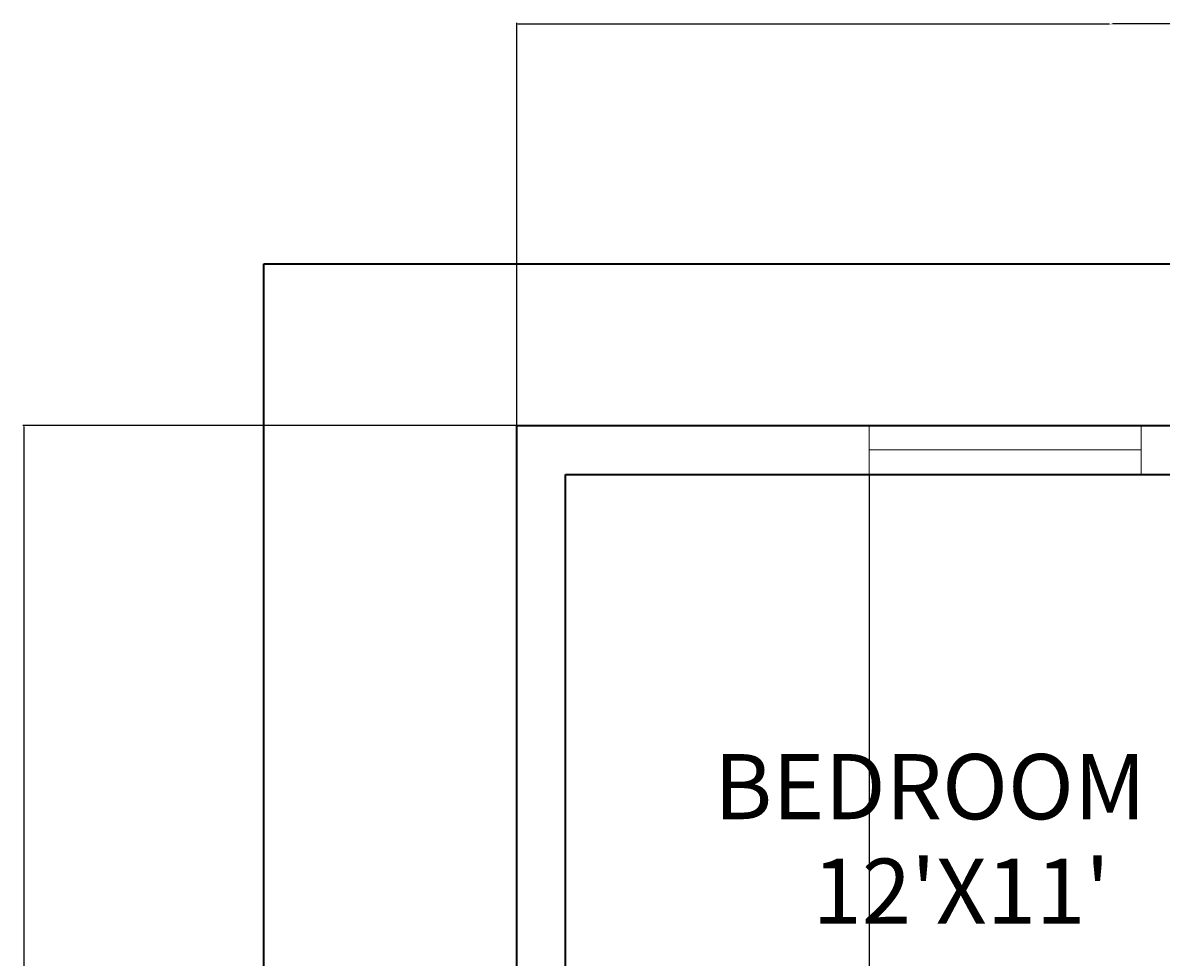
# Model space of a CAD drawing. Units: feet. Extents: x 2100 to 2836, y 2433 to 3396.
# Tile 8 of 12: x 2100 to 2309, y 3224 to 3396. Entities that reach past the tile are written whole.
import ezdxf

# ---------------------------------------------------------------- set-up
doc = ezdxf.new("R2010")
doc.units = ezdxf.units.FT
for name, color, linetype, lineweight in [('A-ANNO-DIMS', 2, 'Continuous', 18), ('A-ANNO-TTLB', 7, 'Continuous', 35), ('A-AREA-IDEN', 7, 'Continuous', 18), ('A-GLAZ', 4, 'Continuous', 18), ('A-WALL', 7, 'Continuous', 35)]:
    doc.layers.add(name, color=color, linetype=linetype, lineweight=lineweight)
doc.styles.get("Standard").update_dxf_attribs({"font": 'arial.ttf'})
doc.dimstyles.get("Standard").update_dxf_attribs({"dimtxt": 0.18, "dimasz": 0.18, "dimexe": 0.18, "dimexo": 0.0625, "dimgap": 0.09, "dimtad": 0, "dimtih": 1, "dimtoh": 1, "dimdec": 4, "dimzin": 0, "dimdsep": 46, "dimtxsty": 'Standard', "dimcen": 0.09, "dimadec": 0, "dimazin": 0, "dimtfac": 1, "dimtdec": 4, "dimtofl": 0, "dimtmove": 0, "dimatfit": 3, "dimfxl": 1, "dimtolj": 1, "dimtzin": 0, "dimarcsym": 0})

# ---------------------------------------------------------------- blocks, each defined once
blk = doc.blocks.new('WIN-REAR-BEDROOM')
for p, q in [((0, 0), (0, 9)), ((50.16, 0), (50.16, 9)), ((0, 4.5), (50.16, 4.5))]:
    blk.add_line(p, q)
blk = doc.blocks.new('*D40')
at = {"layer": 'A-ANNO-DIMS', "color": 0, "lineweight": -2, "transparency": 16777216}
for p, q in [((2190.69, 3321.87), (2190.69, 3396.05)), ((2190.87, 3395.87), (2299.9, 3395.87)), ((2409.51, 3395.87), (2300.48, 3395.87)), ((2409.69, 3321.87), (2409.69, 3396.05))]:
    blk.add_line(p, q, dxfattribs=at)
at = {"layer": 'A-ANNO-DIMS', "color": 0, "transparency": 16777216}
for points in [[(2190.87, 3395.9), (2190.87, 3395.84), (2190.69, 3395.87)], [(2409.51, 3395.9), (2409.51, 3395.84), (2409.69, 3395.87)]]:
    blk.add_solid(points, dxfattribs=at)
at = {"layer": 'Defpoints', "color": 0, "transparency": 16777216}
for p in [(2409.69, 3395.87), (2190.69, 3321.8), (2409.69, 3321.8)]:
    blk.add_point(p, dxfattribs=at)
at = {"layer": 'A-ANNO-DIMS', "color": 0, "transparency": 16777216, "insert": (2300.19, 3395.87), "char_height": 0.18, "attachment_point": 5}
blk.add_mtext('\\A1;219', dxfattribs=at)
blk = doc.blocks.new('*D41')
at = {"layer": 'A-ANNO-DIMS', "color": 0, "lineweight": -2, "transparency": 16777216}
for p, q in [((2190.62, 3321.8), (2099.65, 3321.8)), ((2099.83, 3321.62), (2099.83, 2929.96)), ((2099.83, 2537.94), (2099.83, 2929.6)), ((2190.62, 2537.76), (2099.65, 2537.76))]:
    blk.add_line(p, q, dxfattribs=at)
at = {"layer": 'A-ANNO-DIMS', "color": 0, "transparency": 16777216}
for points in [[(2099.8, 3321.62), (2099.86, 3321.62), (2099.83, 3321.8)], [(2099.8, 2537.94), (2099.86, 2537.94), (2099.83, 2537.76)]]:
    blk.add_solid(points, dxfattribs=at)
at = {"layer": 'Defpoints', "color": 0, "transparency": 16777216}
for p in [(2099.83, 3321.8), (2190.69, 3321.8), (2190.69, 2537.76)]:
    blk.add_point(p, dxfattribs=at)
at = {"layer": 'A-ANNO-DIMS', "color": 0, "transparency": 16777216, "insert": (2099.83, 2929.78), "char_height": 0.18, "attachment_point": 5}
blk.add_mtext('\\A1;784', dxfattribs=at)
blk = doc.blocks.new('*D44')
at = {"layer": 'A-ANNO-DIMS', "color": 0, "lineweight": -2, "transparency": 16777216}
for p, q in [((2199.69, 3312.74), (2199.69, 2433.01)), ((2255.63, 3312.74), (2255.63, 2433.01)), ((2199.87, 2433.19), (2227.26, 2433.19)), ((2255.45, 2433.19), (2228.05, 2433.19))]:
    blk.add_line(p, q, dxfattribs=at)
at = {"layer": 'A-ANNO-DIMS', "color": 0, "transparency": 16777216}
for points in [[(2199.87, 2433.22), (2199.87, 2433.16), (2199.69, 2433.19)], [(2255.45, 2433.22), (2255.45, 2433.16), (2255.63, 2433.19)]]:
    blk.add_solid(points, dxfattribs=at)
at = {"layer": 'Defpoints', "color": 0, "transparency": 16777216}
for p in [(2199.69, 3312.8), (2255.63, 3312.8), (2255.63, 2433.19)]:
    blk.add_point(p, dxfattribs=at)
at = {"layer": 'A-ANNO-DIMS', "color": 0, "transparency": 16777216, "insert": (2227.66, 2433.19), "char_height": 0.18, "attachment_point": 5}
blk.add_mtext('\\A1;55.94', dxfattribs=at)

msp = doc.modelspace()

# ---------------------------------------------------------------- linework, layer by layer
at = {"layer": 'A-ANNO-TTLB'}
msp.add_lwpolyline([(2144.0848, 3351.6245), (2791.0561, 3351.6245), (2791.0561, 2477.4373), (2144.0848, 2477.4373)], close=True, dxfattribs=at)
at = {"layer": 'A-WALL'}
for p, q in [((2190.6857, 3321.8031), (2343.6857, 3321.8031)), ((2190.6857, 2593.755), (2190.6857, 3321.8031)), ((2190.6857, 3321.8031), (2409.6857, 3321.8031)), ((2199.6857, 3312.8031), (2343.6857, 3312.8031)), ((2199.6857, 2905.8031), (2199.6857, 3312.8031))]:
    msp.add_line(p, q, dxfattribs=at)

# ---------------------------------------------------------------- block references
at = {"layer": 'A-GLAZ'}
msp.add_blockref('WIN-REAR-BEDROOM', (2255.625, 3312.8031), dxfattribs=at)

# ---------------------------------------------------------------- texts
at = {"layer": 'A-AREA-IDEN'}
for s, p in [('BEDROOM', (2227.014, 3249.253)), ("12'X11'", (2245.1907, 3229.9761))]:
    msp.add_text(s, height=12, dxfattribs=at).set_placement(p)

# ---------------------------------------------------------------- dimensions: what is measured, and where the dimension line sits
at = {"layer": 'A-ANNO-DIMS'}
for base, p1, p2, override, picture, middle in [((2409.6857, 3395.8745), (2190.6857, 3321.8031), (2409.6857, 3321.8031), {"dimdec": 0, "dimlfac": 1, "dimrnd": 0, "dimzin": 0, "dimdsep": 46, "dimlunit": 2}, '*D40', (2300.1857, 3395.8745)), ((2255.625, 2433.1873), (2199.6857, 3312.8031), (2255.625, 3312.8031), {"dimdec": 2, "dimlfac": 1, "dimrnd": 0, "dimzin": 0, "dimdsep": 46, "dimlunit": 2}, '*D44', (2227.6554, 2433.1873))]:
    dim = msp.add_linear_dim(base=base, p1=p1, p2=p2, dimstyle='Standard', override=override, dxfattribs=at)
    dim.commit()
    dim.dimension.update_dxf_attribs({"geometry": picture, "text_midpoint": middle})
dim = msp.add_linear_dim(base=(2099.8348, 3321.8031), p1=(2190.6857, 2537.755), p2=(2190.6857, 3321.8031), angle=90, dimstyle='Standard', override={"dimdec": 0, "dimlfac": 1, "dimrnd": 0, "dimzin": 0, "dimdsep": 46, "dimlunit": 2}, dxfattribs=at)
dim.commit()
dim.dimension.update_dxf_attribs({"geometry": '*D41', "text_midpoint": (2099.8348, 2929.7791)})

doc.saveas('drawing.dxf')
